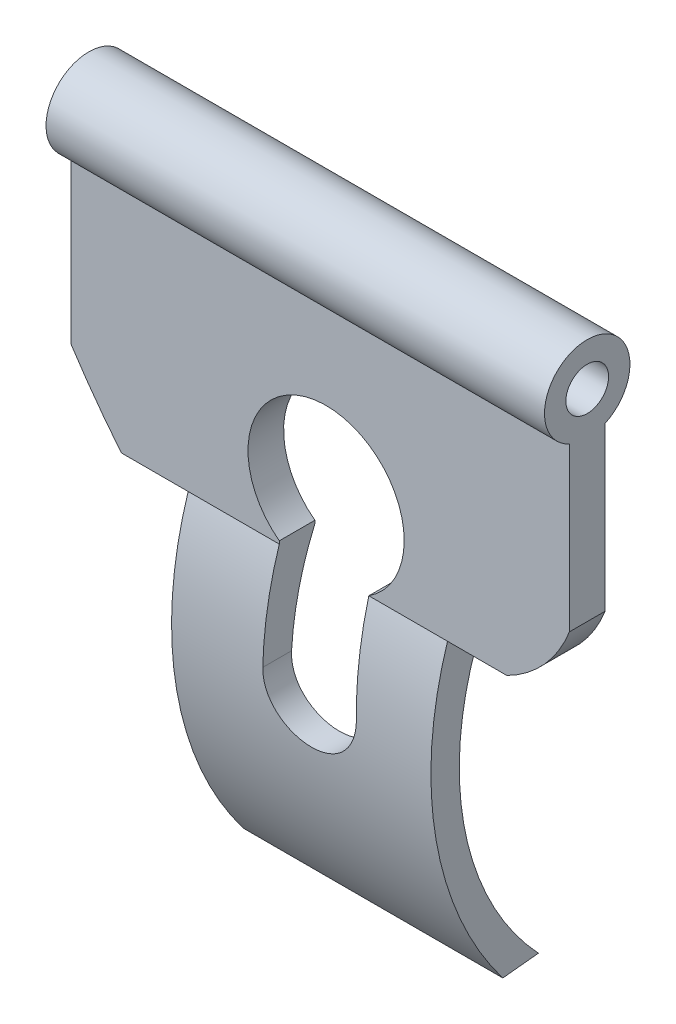
ISO-10303-21;
HEADER;
FILE_DESCRIPTION(('STEP AP214'),'2;1');
FILE_NAME('part.step','',(''),(''),'','','');
FILE_SCHEMA(('AUTOMOTIVE_DESIGN { 1 0 10303 214 1 1 1 1 }'));
ENDSEC;
DATA;
#1=APPLICATION_CONTEXT('core data for automotive mechanical design processes');
#2=APPLICATION_PROTOCOL_DEFINITION('international standard','automotive_design',2000,#1);
#3=PRODUCT_CONTEXT('',#1,'mechanical');
#4=PRODUCT('Part','Part','',(#3));
#5=PRODUCT_RELATED_PRODUCT_CATEGORY('part','',(#4));
#6=PRODUCT_DEFINITION_FORMATION('','',#4);
#7=PRODUCT_DEFINITION_CONTEXT('part definition',#1,'design');
#8=PRODUCT_DEFINITION('design','',#6,#7);
#9=PRODUCT_DEFINITION_SHAPE('','',#8);
#10=(LENGTH_UNIT() NAMED_UNIT(*) SI_UNIT(.MILLI.,.METRE.));
#11=(NAMED_UNIT(*) PLANE_ANGLE_UNIT() SI_UNIT($,.RADIAN.));
#12=(NAMED_UNIT(*) SI_UNIT($,.STERADIAN.) SOLID_ANGLE_UNIT());
#13=UNCERTAINTY_MEASURE_WITH_UNIT(LENGTH_MEASURE(1.E-05),#10,'distance_accuracy_value','');
#14=(GEOMETRIC_REPRESENTATION_CONTEXT(3) GLOBAL_UNCERTAINTY_ASSIGNED_CONTEXT((#13)) GLOBAL_UNIT_ASSIGNED_CONTEXT((#10,
#11,#12)) REPRESENTATION_CONTEXT('',''));
#15=CARTESIAN_POINT('',(0.,0.,0.));
#16=DIRECTION('',(0.,0.,1.));
#17=DIRECTION('',(1.,0.,0.));
#18=AXIS2_PLACEMENT_3D('',#15,#16,#17);
#19=CARTESIAN_POINT('',(6.99999999999999,-52.9712864227578,-44.3974159261056));
#20=DIRECTION('',(1.,0.,0.));
#21=DIRECTION('',(0.,0.,-1.));
#22=AXIS2_PLACEMENT_3D('',#19,#20,#21);
#23=CYLINDRICAL_SURFACE('',#22,49.2291279396497);
#24=CARTESIAN_POINT('',(42.4478068961798,-52.9712864227578,-44.3974159261056));
#25=DIRECTION('',(0.999136886042049,0.0415389329448733,0.));
#26=DIRECTION('',(0.0415389329448733,-0.999136886042049,0.));
#27=AXIS2_PLACEMENT_3D('',#24,#25,#26);
#28=ELLIPSE('',#27,49.2716549928054,49.2291279396497);
#29=CARTESIAN_POINT('',(42.4004064881789,-51.8311633456915,4.81850788994741));
#30=VERTEX_POINT('',#29);
#31=CARTESIAN_POINT('',(41.8253784066492,-38.,2.5));
#32=VERTEX_POINT('',#31);
#33=EDGE_CURVE('E182',#30,#32,#28,.F.);
#34=ORIENTED_EDGE('',*,*,#33,.F.);
#35=CARTESIAN_POINT('',(42.4004064881789,-51.8311633456915,4.81850788994741));
#36=CARTESIAN_POINT('',(42.4004272866516,-52.0148228202435,4.82277278769377));
#37=CARTESIAN_POINT('',(42.3927093008387,-52.1985036306068,4.82598935199668));
#38=CARTESIAN_POINT('',(42.3619341165299,-52.5645884625414,4.83036962650464));
#39=CARTESIAN_POINT('',(42.3388779445284,-52.7469925687296,4.83153347406691));
#40=CARTESIAN_POINT('',(42.2775957275639,-53.1090462090531,4.83185252541183));
#41=CARTESIAN_POINT('',(42.2393850548384,-53.2886983434919,4.8310097603167));
#42=CARTESIAN_POINT('',(42.1480749260284,-53.644156459105,4.82743406908749));
#43=CARTESIAN_POINT('',(42.0949756075018,-53.8199624757978,4.82470116041634));
#44=CARTESIAN_POINT('',(41.9742581345645,-54.1665174469575,4.81750572105998));
#45=CARTESIAN_POINT('',(41.906637220099,-54.3372654330369,4.81304286144073));
#46=CARTESIAN_POINT('',(41.7573422013104,-54.6725294681309,4.80259373184012));
#47=CARTESIAN_POINT('',(41.6756629058677,-54.837043187637,4.79660689873226));
#48=CARTESIAN_POINT('',(41.4988942693706,-55.1585452676515,4.78336094522803));
#49=CARTESIAN_POINT('',(41.4038112649323,-55.3155371374003,4.77610242563115));
#50=CARTESIAN_POINT('',(41.2008420968024,-55.6210450901704,4.76058671666513));
#51=CARTESIAN_POINT('',(41.0929511910275,-55.7695580035581,4.75232915738302));
#52=CARTESIAN_POINT('',(40.8647093433168,-56.0575769758064,4.73508601210607));
#53=CARTESIAN_POINT('',(40.7443116463755,-56.1970458223169,4.72609772372094));
#54=CARTESIAN_POINT('',(40.4922042135143,-56.465423999144,4.70773800860886));
#55=CARTESIAN_POINT('',(40.360490315565,-56.5943294099422,4.69836644158412));
#56=CARTESIAN_POINT('',(40.0867365556308,-56.8406018513904,4.67957143470314));
#57=CARTESIAN_POINT('',(39.9446988003194,-56.9579712246355,4.67014800579052));
#58=CARTESIAN_POINT('',(39.6512082833703,-57.1804235682722,4.65156641941204));
#59=CARTESIAN_POINT('',(39.4997520621253,-57.2855019826076,4.64240836125511));
#60=CARTESIAN_POINT('',(39.1878509828328,-57.4830116330515,4.62463270633958));
#61=CARTESIAN_POINT('',(39.0273699928713,-57.5753860471284,4.61601762558071));
#62=CARTESIAN_POINT('',(38.6990917364206,-57.7463173568394,4.5996604727672));
#63=CARTESIAN_POINT('',(38.5312917779282,-57.8248691139358,4.59191872575443));
#64=CARTESIAN_POINT('',(38.1896957883277,-57.967513154658,4.57757663028869));
#65=CARTESIAN_POINT('',(38.015902492014,-58.0316119351845,4.57097576929753));
#66=CARTESIAN_POINT('',(37.6634195132357,-58.1449479231074,4.55913128898036));
#67=CARTESIAN_POINT('',(37.4847280619881,-58.194179682624,4.55388816728516));
#68=CARTESIAN_POINT('',(37.1244168317102,-58.2772419705253,4.54495441141868));
#69=CARTESIAN_POINT('',(36.9428093788423,-58.3111253962825,4.54125844842583));
#70=CARTESIAN_POINT('',(36.577357970659,-58.3634916039002,4.53551630242693));
#71=CARTESIAN_POINT('',(36.3935139773426,-58.3819741237124,4.53347014749256));
#72=CARTESIAN_POINT('',(36.0249142215589,-58.4033999645648,4.53109618096684));
#73=CARTESIAN_POINT('',(35.8401584720371,-58.4063435055996,4.5307683450482));
#74=CARTESIAN_POINT('',(35.4710601094936,-58.3966700205534,4.53184192656726));
#75=CARTESIAN_POINT('',(35.2867174954444,-58.3840530332211,4.53324333969879));
#76=CARTESIAN_POINT('',(34.9206400396917,-58.3434492359607,4.53771785216521));
#77=CARTESIAN_POINT('',(34.738896974958,-58.3155356332202,4.54078298852421));
#78=CARTESIAN_POINT('',(34.3784227433714,-58.2445940203224,4.54847803563724));
#79=CARTESIAN_POINT('',(34.1996915178474,-58.2015663049481,4.55310791587269));
#80=CARTESIAN_POINT('',(33.8464638134781,-58.1006997626879,4.56378020106195));
#81=CARTESIAN_POINT('',(33.6719681832891,-58.0428579939984,4.56982288655258));
#82=CARTESIAN_POINT('',(33.3285355356356,-57.9128086743332,4.58311758350949));
#83=CARTESIAN_POINT('',(33.1595965372608,-57.8406063089645,4.5903691582937));
#84=CARTESIAN_POINT('',(32.8279446328418,-57.6821255333204,4.60586340056811));
#85=CARTESIAN_POINT('',(32.6652496427565,-57.5958098858852,4.61410867432524));
#86=CARTESIAN_POINT('',(32.3477591459481,-57.4098873761342,4.63129573700929));
#87=CARTESIAN_POINT('',(32.1929607941153,-57.3102853482478,4.64023727210181));
#88=CARTESIAN_POINT('',(31.8922216245507,-57.0984279798047,4.65852198288474));
#89=CARTESIAN_POINT('',(31.7462839968443,-56.9861681232656,4.66786530118074));
#90=CARTESIAN_POINT('',(31.4643920486273,-56.7498511970862,4.6866296035705));
#91=CARTESIAN_POINT('',(31.3284341113722,-56.6257984390994,4.69605055813751));
#92=CARTESIAN_POINT('',(31.0666656532321,-56.3660050605062,4.71470041689289));
#93=CARTESIAN_POINT('',(30.9409154211626,-56.2302035855989,4.72392797053744));
#94=CARTESIAN_POINT('',(30.701338784207,-55.9485123735807,4.7418053591569));
#95=CARTESIAN_POINT('',(30.5875080032234,-55.8026263717834,4.75045540573158));
#96=CARTESIAN_POINT('',(30.3724563320646,-55.501646336587,4.76687030854798));
#97=CARTESIAN_POINT('',(30.2712437324657,-55.3465463470523,4.77463458252535));
#98=CARTESIAN_POINT('',(30.0822783794528,-55.0283789273214,4.78897195642646));
#99=CARTESIAN_POINT('',(29.9945205696038,-54.8653145207552,4.79554550400561));
#100=CARTESIAN_POINT('',(29.8330944341739,-54.5324023606024,4.80723506652109));
#101=CARTESIAN_POINT('',(29.7594192644044,-54.3625579508767,4.81235179007149));
#102=CARTESIAN_POINT('',(29.6266685443386,-54.0172880049236,4.82090102153776));
#103=CARTESIAN_POINT('',(29.5675874145293,-53.8418646306581,4.82433417360352));
#104=CARTESIAN_POINT('',(29.4644758401622,-53.4868264235191,4.82933232381355));
#105=CARTESIAN_POINT('',(29.4204296685412,-53.3072161817153,4.83089927836055));
#106=CARTESIAN_POINT('',(29.3476402120207,-52.9449884342697,4.83203788223034));
#107=CARTESIAN_POINT('',(29.3188895924397,-52.7623724133808,4.83161048886596));
#108=CARTESIAN_POINT('',(29.2836563472731,-52.4546973770444,4.8291583095));
#109=CARTESIAN_POINT('',(29.2729807758379,-52.3300980785225,4.82769402379001));
#110=CARTESIAN_POINT('',(29.2587610500021,-52.0807206316672,4.8238142284511));
#111=CARTESIAN_POINT('',(29.2552048011394,-51.9559431476322,4.8214003403914));
#112=CARTESIAN_POINT('',(29.255207416721,-51.8311633456915,4.8185078899474));
#113=B_SPLINE_CURVE_WITH_KNOTS('',3,(#35,#36,#37,#38,#39,#40,#41,#42,#43,#44,#45,#46,#47,#48,
#49,#50,#51,#52,#53,#54,#55,#56,#57,#58,#59,#60,#61,#62,#63,#64,#65,#66,#67,#68,#69,#70,#71,#72,
#73,#74,#75,#76,#77,#78,#79,#80,#81,#82,#83,#84,#85,#86,#87,#88,#89,#90,#91,#92,#93,#94,#95,#96,
#97,#98,#99,#100,#101,#102,#103,#104,#105,#106,#107,#108,#109,#110,#111,#112),.UNSPECIFIED.,.F.,
.F.,(4,2,2,2,2,2,2,2,2,2,2,2,2,2,2,2,2,2,2,2,2,2,2,2,2,2,2,2,2,2,2,2,2,2,2,2,2,2,4),(0.,
0.550957649228606,1.10187842981338,1.65224179756538,2.2026000806112,2.7530630605223,
3.30372973912141,3.85413695716424,4.4047486010136,4.95749824290263,5.51045206022659,
6.063293357563,6.61633893895976,7.17178286448609,7.72743284066219,8.28283254093139,
8.83843551591308,9.39210878152291,9.94579146775293,10.4994663151433,11.0531397837793,
11.6041863110236,12.1552220913444,12.7063673823802,13.2573140151696,13.8097384706839,
14.3619624645968,14.9143841047404,15.4666045427803,16.0218795128123,16.5769498995431,
17.1323830856685,17.6876070204661,18.2425604254873,18.7973013342543,19.3514601745986,
19.9053530388913,20.2803524190753,20.6547141996082),.UNSPECIFIED.);
#114=CARTESIAN_POINT('',(29.255207416721,-51.8311633456915,4.81850788994741));
#115=VERTEX_POINT('',#114);
#116=EDGE_CURVE('E167',#30,#115,#113,.T.);
#117=ORIENTED_EDGE('',*,*,#116,.T.);
#118=CARTESIAN_POINT('',(29.255207416721,-52.9712864227578,-44.3974159261056));
#119=DIRECTION('',(1.,0.,0.));
#120=DIRECTION('',(0.,0.,-1.));
#121=AXIS2_PLACEMENT_3D('',#118,#119,#120);
#122=CIRCLE('',#121,49.2291279396497);
#123=CARTESIAN_POINT('',(29.255207416721,-38.,2.5));
#124=VERTEX_POINT('',#123);
#125=EDGE_CURVE('E166',#115,#124,#122,.F.);
#126=ORIENTED_EDGE('',*,*,#125,.T.);
#127=DIRECTION('',(-1.,0.,0.));
#128=VECTOR('',#127,1.);
#129=CARTESIAN_POINT('',(70.,-38.,2.5));
#130=LINE('',#129,#128);
#131=CARTESIAN_POINT('',(16.4571242651207,-38.,2.5));
#132=VERTEX_POINT('',#131);
#133=EDGE_CURVE('E170',#124,#132,#130,.T.);
#134=ORIENTED_EDGE('',*,*,#133,.T.);
#135=CARTESIAN_POINT('',(16.4571242651207,-52.9712864227578,-44.3974159261056));
#136=DIRECTION('',(-1.,0.,0.));
#137=DIRECTION('',(0.,0.,1.));
#138=AXIS2_PLACEMENT_3D('',#135,#136,#137);
#139=CIRCLE('',#138,49.2291279396497);
#140=CARTESIAN_POINT('',(16.4571242651207,-82.841381432004,-5.26578598513591));
#141=VERTEX_POINT('',#140);
#142=EDGE_CURVE('E243',#132,#141,#139,.F.);
#143=ORIENTED_EDGE('',*,*,#142,.T.);
#144=DIRECTION('',(1.,0.,0.));
#145=VECTOR('',#144,1.);
#146=CARTESIAN_POINT('',(6.99999999999999,-82.841381432004,-5.26578598513591));
#147=LINE('',#146,#145);
#148=CARTESIAN_POINT('',(52.8806301729192,-82.841381432004,-5.26578598513591));
#149=VERTEX_POINT('',#148);
#150=EDGE_CURVE('E261',#141,#149,#147,.T.);
#151=ORIENTED_EDGE('',*,*,#150,.T.);
#152=CARTESIAN_POINT('',(52.8806301729192,-52.9712864227578,-44.3974159261056));
#153=DIRECTION('',(1.,0.,0.));
#154=DIRECTION('',(0.,0.,-1.));
#155=AXIS2_PLACEMENT_3D('',#152,#153,#154);
#156=CIRCLE('',#155,49.2291279396497);
#157=CARTESIAN_POINT('',(52.8806301729192,-38.,2.49999999999999));
#158=VERTEX_POINT('',#157);
#159=EDGE_CURVE('E256',#149,#158,#156,.F.);
#160=ORIENTED_EDGE('',*,*,#159,.T.);
#161=EDGE_CURVE('E231',#158,#32,#130,.T.);
#162=ORIENTED_EDGE('',*,*,#161,.T.);
#163=EDGE_LOOP('',(#34,#117,#126,#134,#143,#151,#160,#162));
#164=FACE_BOUND('',#163,.T.);
#165=ADVANCED_FACE('F45',(#164),#23,.T.);
#166=CARTESIAN_POINT('',(6.99999999999999,-54.237018869758,-40.2033993287331));
#167=DIRECTION('',(1.,0.,0.));
#168=DIRECTION('',(0.,0.,-1.));
#169=AXIS2_PLACEMENT_3D('',#166,#167,#168);
#170=CYLINDRICAL_SURFACE('',#169,41.0510304708517);
#171=CARTESIAN_POINT('',(42.5004294907178,-54.237018869758,-40.2033993287331));
#172=DIRECTION('',(0.999136886042049,0.0415389329448733,0.));
#173=DIRECTION('',(0.0415389329448733,-0.999136886042049,0.));
#174=AXIS2_PLACEMENT_3D('',#171,#172,#173);
#175=ELLIPSE('',#174,41.0864927962674,41.0510304708517);
#176=CARTESIAN_POINT('',(41.8253784066492,-38.,-2.5));
#177=VERTEX_POINT('',#176);
#178=CARTESIAN_POINT('',(42.4004064881789,-51.8311633456915,0.777071165346227));
#179=VERTEX_POINT('',#178);
#180=EDGE_CURVE('E12',#177,#179,#175,.T.);
#181=ORIENTED_EDGE('',*,*,#180,.F.);
#182=DIRECTION('',(-1.,0.,0.));
#183=VECTOR('',#182,1.);
#184=CARTESIAN_POINT('',(70.,-38.,-2.5));
#185=LINE('',#184,#183);
#186=CARTESIAN_POINT('',(52.8806301729192,-38.,-2.5));
#187=VERTEX_POINT('',#186);
#188=EDGE_CURVE('E314',#187,#177,#185,.T.);
#189=ORIENTED_EDGE('',*,*,#188,.F.);
#190=CARTESIAN_POINT('',(52.8806301729192,-54.237018869758,-40.2033993287331));
#191=DIRECTION('',(1.,0.,0.));
#192=DIRECTION('',(0.,0.,-1.));
#193=AXIS2_PLACEMENT_3D('',#190,#191,#192);
#194=CIRCLE('',#193,41.0510304708517);
#195=CARTESIAN_POINT('',(52.8806301729192,-82.3248527130443,-10.2657859851359));
#196=VERTEX_POINT('',#195);
#197=EDGE_CURVE('E257',#187,#196,#194,.T.);
#198=ORIENTED_EDGE('',*,*,#197,.T.);
#199=DIRECTION('',(1.,0.,0.));
#200=VECTOR('',#199,1.);
#201=CARTESIAN_POINT('',(6.99999999999999,-82.3248527130443,-10.2657859851359));
#202=LINE('',#201,#200);
#203=CARTESIAN_POINT('',(16.4571242651207,-82.3248527130443,-10.2657859851359));
#204=VERTEX_POINT('',#203);
#205=EDGE_CURVE('E265',#204,#196,#202,.T.);
#206=ORIENTED_EDGE('',*,*,#205,.F.);
#207=CARTESIAN_POINT('',(16.4571242651207,-54.237018869758,-40.2033993287331));
#208=DIRECTION('',(-1.,0.,0.));
#209=DIRECTION('',(0.,0.,1.));
#210=AXIS2_PLACEMENT_3D('',#207,#208,#209);
#211=CIRCLE('',#210,41.0510304708517);
#212=CARTESIAN_POINT('',(16.4571242651207,-38.,-2.5));
#213=VERTEX_POINT('',#212);
#214=EDGE_CURVE('E238',#204,#213,#211,.T.);
#215=ORIENTED_EDGE('',*,*,#214,.T.);
#216=CARTESIAN_POINT('',(29.255207416721,-38.,-2.5));
#217=VERTEX_POINT('',#216);
#218=EDGE_CURVE('E311',#217,#213,#185,.T.);
#219=ORIENTED_EDGE('',*,*,#218,.F.);
#220=CARTESIAN_POINT('',(29.255207416721,-54.237018869758,-40.2033993287331));
#221=DIRECTION('',(1.,0.,0.));
#222=DIRECTION('',(0.,0.,-1.));
#223=AXIS2_PLACEMENT_3D('',#220,#221,#222);
#224=CIRCLE('',#223,41.0510304708517);
#225=CARTESIAN_POINT('',(29.255207416721,-51.8311633456915,0.777071165346227));
#226=VERTEX_POINT('',#225);
#227=EDGE_CURVE('E151',#217,#226,#224,.T.);
#228=ORIENTED_EDGE('',*,*,#227,.T.);
#229=CARTESIAN_POINT('',(29.255207416721,-51.8311633456915,0.777071165346227));
#230=CARTESIAN_POINT('',(29.2551862710845,-52.013900503685,0.78781138328913));
#231=CARTESIAN_POINT('',(29.2628275127138,-52.1967096143398,0.797305349333378));
#232=CARTESIAN_POINT('',(29.2933189270613,-52.5611583890662,0.81381167871571));
#233=CARTESIAN_POINT('',(29.3161683031272,-52.7427981138909,0.820824172012072));
#234=CARTESIAN_POINT('',(29.3769285798627,-53.1034267161399,0.832373576017649));
#235=CARTESIAN_POINT('',(29.4148238051525,-53.28241815198,0.836913051578508));
#236=CARTESIAN_POINT('',(29.5054125969348,-53.6366582211059,0.843622917104425));
#237=CARTESIAN_POINT('',(29.5581059482637,-53.8119069087711,0.845793341513061));
#238=CARTESIAN_POINT('',(29.6779396610719,-54.1574584384914,0.847917845102459));
#239=CARTESIAN_POINT('',(29.7450838406128,-54.3277599599303,0.847871337829038));
#240=CARTESIAN_POINT('',(29.8933611044865,-54.6622218276805,0.845769788062237));
#241=CARTESIAN_POINT('',(29.9744993622682,-54.8263798754096,0.84371400144515));
#242=CARTESIAN_POINT('',(30.1501275580187,-55.147253954466,0.83785206132433));
#243=CARTESIAN_POINT('',(30.2446110229159,-55.3039735448552,0.834046754416508));
#244=CARTESIAN_POINT('',(30.4463275536636,-55.6090188799371,0.824981281851952));
#245=CARTESIAN_POINT('',(30.5535653485026,-55.7573414809606,0.819720575604585));
#246=CARTESIAN_POINT('',(30.7803890031573,-56.0449853991545,0.80805215323785));
#247=CARTESIAN_POINT('',(30.9000151196575,-56.1842748165466,0.801640644673474));
#248=CARTESIAN_POINT('',(31.1505215353129,-56.4523902713932,0.788029795262536));
#249=CARTESIAN_POINT('',(31.2814059674549,-56.5812124322238,0.780830164825596));
#250=CARTESIAN_POINT('',(31.553453057285,-56.827423405374,0.766005340486057));
#251=CARTESIAN_POINT('',(31.6946138151236,-56.9448143217266,0.758380225306077));
#252=CARTESIAN_POINT('',(31.9863091073212,-57.1674196595499,0.743057296638023));
#253=CARTESIAN_POINT('',(32.1368470932725,-57.2726295561806,0.7353594572765));
#254=CARTESIAN_POINT('',(32.4472830811458,-57.4707791264487,0.720186094246282));
#255=CARTESIAN_POINT('',(32.6072388571895,-57.5636284526595,0.712712487196203));
#256=CARTESIAN_POINT('',(32.9344863346986,-57.7355630844579,0.698370070397983));
#257=CARTESIAN_POINT('',(33.1017807371311,-57.8146432682162,0.691501486172938));
#258=CARTESIAN_POINT('',(33.4423942049698,-57.9583997671651,0.678670531490853));
#259=CARTESIAN_POINT('',(33.615710561302,-58.0230824647396,0.672707759862171));
#260=CARTESIAN_POINT('',(33.9672751487667,-58.1376424527887,0.66193503747772));
#261=CARTESIAN_POINT('',(34.145525162996,-58.1875143119637,0.657125509753563));
#262=CARTESIAN_POINT('',(34.5053643027338,-58.2719952625799,0.648869509439004));
#263=CARTESIAN_POINT('',(34.6869482088694,-58.306626391512,0.645421069519342));
#264=CARTESIAN_POINT('',(35.0524127875527,-58.3604776304912,0.640020270305216));
#265=CARTESIAN_POINT('',(35.2362935009873,-58.3796974657934,0.638067937682636));
#266=CARTESIAN_POINT('',(35.6050284821548,-58.4025830095945,0.635740122710671));
#267=CARTESIAN_POINT('',(35.7898827400214,-58.4062488754214,0.635364624411638));
#268=CARTESIAN_POINT('',(36.1592393085816,-58.3979997301201,0.636205934242317));
#269=CARTESIAN_POINT('',(36.343741620223,-58.3860847610079,0.637422738078154));
#270=CARTESIAN_POINT('',(36.7102636078965,-58.3468486871214,0.64138965420686));
#271=CARTESIAN_POINT('',(36.8922906271707,-58.3195954488421,0.64413301143375));
#272=CARTESIAN_POINT('',(37.2533895140513,-58.2499318982601,0.651035620126144));
#273=CARTESIAN_POINT('',(37.4324614393567,-58.2075218822654,0.655194843912049));
#274=CARTESIAN_POINT('',(37.7864248537003,-58.1078419353391,0.664758644976362));
#275=CARTESIAN_POINT('',(37.9613154929022,-58.0505690111321,0.670163473085332));
#276=CARTESIAN_POINT('',(38.3055876978027,-57.9216021047379,0.681990937307442));
#277=CARTESIAN_POINT('',(38.4749712309712,-57.8499133400098,0.68841320500543));
#278=CARTESIAN_POINT('',(38.8075294105995,-57.6924135404842,0.702023417913938));
#279=CARTESIAN_POINT('',(38.97068741417,-57.6065675271036,0.709213243625769));
#280=CARTESIAN_POINT('',(39.2891450120115,-57.4215216268564,0.724032215094351));
#281=CARTESIAN_POINT('',(39.4444474485978,-57.3223266181928,0.731661199786547));
#282=CARTESIAN_POINT('',(39.7462296118795,-57.1112155047978,0.747025538856692));
#283=CARTESIAN_POINT('',(39.8927061201492,-56.9992948020074,0.754760930788738));
#284=CARTESIAN_POINT('',(40.1756998498758,-56.7635857505098,0.769976175345955));
#285=CARTESIAN_POINT('',(40.3122207085268,-56.639801774565,0.77745612075947));
#286=CARTESIAN_POINT('',(40.5749846796514,-56.3806218370759,0.791831897448136));
#287=CARTESIAN_POINT('',(40.7011798291845,-56.2451770896073,0.798725008271243));
#288=CARTESIAN_POINT('',(40.941675288446,-55.9641532633959,0.811523342643876));
#289=CARTESIAN_POINT('',(41.0559800066479,-55.8185779742841,0.817428932821558));
#290=CARTESIAN_POINT('',(41.2719962201283,-55.5181829706114,0.827909656277159));
#291=CARTESIAN_POINT('',(41.3736998996042,-55.3633576060434,0.832483966176567));
#292=CARTESIAN_POINT('',(41.5636598666664,-55.0457067379401,0.839972264079861));
#293=CARTESIAN_POINT('',(41.6519212581197,-54.8828843020023,0.842886883404363));
#294=CARTESIAN_POINT('',(41.8141458541011,-54.5508766999773,0.846765919768479));
#295=CARTESIAN_POINT('',(41.8881530735077,-54.3817131122054,0.84773643013108));
#296=CARTESIAN_POINT('',(42.0216514093965,-54.0378261992285,0.847507766434327));
#297=CARTESIAN_POINT('',(42.0811480986328,-53.8631050376386,0.846309426813219));
#298=CARTESIAN_POINT('',(42.1851828875006,-53.5094875947464,0.841564274849871));
#299=CARTESIAN_POINT('',(42.2297357594675,-53.3305956246509,0.838019792098701));
#300=CARTESIAN_POINT('',(42.3036366062835,-52.9698356260756,0.828464936215655));
#301=CARTESIAN_POINT('',(42.3329916827179,-52.7879690286299,0.822455717156139));
#302=CARTESIAN_POINT('',(42.3699134127951,-52.4766731433532,0.810072284142807));
#303=CARTESIAN_POINT('',(42.3813581031596,-52.3476648360665,0.804333180483692));
#304=CARTESIAN_POINT('',(42.3965997019823,-52.0894839051512,0.791623835013054));
#305=CARTESIAN_POINT('',(42.4004099066028,-51.960311959928,0.784655756650464));
#306=CARTESIAN_POINT('',(42.4004064881789,-51.8311633456915,0.777071165346227));
#307=B_SPLINE_CURVE_WITH_KNOTS('',3,(#229,#230,#231,#232,#233,#234,#235,#236,#237,#238,#239,
#240,#241,#242,#243,#244,#245,#246,#247,#248,#249,#250,#251,#252,#253,#254,#255,#256,#257,#258,
#259,#260,#261,#262,#263,#264,#265,#266,#267,#268,#269,#270,#271,#272,#273,#274,#275,#276,#277,
#278,#279,#280,#281,#282,#283,#284,#285,#286,#287,#288,#289,#290,#291,#292,#293,#294,#295,#296,
#297,#298,#299,#300,#301,#302,#303,#304,#305,#306),.UNSPECIFIED.,.F.,.F.,(4,2,2,2,2,2,2,2,2,2,2,
2,2,2,2,2,2,2,2,2,2,2,2,2,2,2,2,2,2,2,2,2,2,2,2,2,2,2,4),(0.,0.548992098899319,1.09795544204003,
1.64634834725046,2.19473327928324,2.74326327867393,3.29199649963299,3.84046446665669,
4.38913642968264,4.93965088569598,5.49036830808905,6.04098417316574,6.5918039217418,
7.14645136521526,7.7013046870533,8.2559115512132,8.81072154547037,9.36472664932581,
9.91874162948923,10.4727510057888,11.0267588881246,11.5783345353855,12.1298994001926,
12.6815754322438,13.2330521569261,13.7859124202628,14.3385711944416,14.8914302941705,
15.4440863899717,15.9991788812913,16.5540648285068,17.1092932392432,17.6643103083577,
18.2175850764174,18.7706470240916,19.323160633827,19.8754158329254,20.2641235305148,
20.6521536672614),.UNSPECIFIED.);
#308=EDGE_CURVE('E49',#226,#179,#307,.T.);
#309=ORIENTED_EDGE('',*,*,#308,.T.);
#310=EDGE_LOOP('',(#181,#189,#198,#206,#215,#219,#228,#309));
#311=FACE_BOUND('',#310,.T.);
#312=ADVANCED_FACE('F207',(#311),#170,.F.);
#313=CARTESIAN_POINT('',(6.99999999999999,-82.841381432004,-5.26578598513591));
#314=DIRECTION('',(0.,-0.994706295284288,-0.102758873688879));
#315=DIRECTION('',(0.,0.102758873688879,-0.994706295284288));
#316=AXIS2_PLACEMENT_3D('',#313,#314,#315);
#317=PLANE('',#316);
#318=ORIENTED_EDGE('',*,*,#150,.F.);
#319=DIRECTION('',(0.,0.102758873688879,-0.994706295284288));
#320=VECTOR('',#319,1.);
#321=CARTESIAN_POINT('',(16.4571242651207,-82.841381432004,-5.26578598513591));
#322=LINE('',#321,#320);
#323=EDGE_CURVE('E321',#141,#204,#322,.T.);
#324=ORIENTED_EDGE('',*,*,#323,.T.);
#325=ORIENTED_EDGE('',*,*,#205,.T.);
#326=DIRECTION('',(0.,-0.102758873688879,0.994706295284288));
#327=VECTOR('',#326,1.);
#328=CARTESIAN_POINT('',(52.8806301729192,-82.841381432004,-5.26578598513591));
#329=LINE('',#328,#327);
#330=EDGE_CURVE('E322',#196,#149,#329,.T.);
#331=ORIENTED_EDGE('',*,*,#330,.T.);
#332=EDGE_LOOP('',(#318,#324,#325,#331));
#333=FACE_BOUND('',#332,.T.);
#334=ADVANCED_FACE('F208',(#333),#317,.T.);
#335=CARTESIAN_POINT('',(70.,0.,0.));
#336=DIRECTION('',(1.,0.,0.));
#337=DIRECTION('',(0.,0.,-1.));
#338=AXIS2_PLACEMENT_3D('',#335,#336,#337);
#339=PLANE('',#338);
#340=DIRECTION('',(0.,0.,-1.));
#341=VECTOR('',#340,1.);
#342=CARTESIAN_POINT('',(70.,-28.2978126777009,67.5));
#343=LINE('',#342,#341);
#344=CARTESIAN_POINT('',(70.,-28.2978126777009,2.5));
#345=VERTEX_POINT('',#344);
#346=CARTESIAN_POINT('',(70.,-28.2978126777009,-2.5));
#347=VERTEX_POINT('',#346);
#348=EDGE_CURVE('E270',#345,#347,#343,.T.);
#349=ORIENTED_EDGE('',*,*,#348,.T.);
#350=DIRECTION('',(0.,1.,0.));
#351=VECTOR('',#350,1.);
#352=CARTESIAN_POINT('',(70.,-5.45435605731786,-2.5));
#353=LINE('',#352,#351);
#354=CARTESIAN_POINT('',(70.,-5.45435605731786,-2.5));
#355=VERTEX_POINT('',#354);
#356=EDGE_CURVE('E297',#347,#355,#353,.T.);
#357=ORIENTED_EDGE('',*,*,#356,.T.);
#358=CARTESIAN_POINT('',(70.,0.,0.));
#359=DIRECTION('',(1.,0.,0.));
#360=DIRECTION('',(0.,0.,-1.));
#361=AXIS2_PLACEMENT_3D('',#358,#359,#360);
#362=CIRCLE('',#361,6.);
#363=CARTESIAN_POINT('',(70.,-5.45435605731786,2.5));
#364=VERTEX_POINT('',#363);
#365=EDGE_CURVE('E291',#355,#364,#362,.T.);
#366=ORIENTED_EDGE('',*,*,#365,.T.);
#367=DIRECTION('',(0.,-1.,0.));
#368=VECTOR('',#367,1.);
#369=CARTESIAN_POINT('',(70.,-5.45435605731786,2.5));
#370=LINE('',#369,#368);
#371=EDGE_CURVE('E298',#364,#345,#370,.T.);
#372=ORIENTED_EDGE('',*,*,#371,.T.);
#373=EDGE_LOOP('',(#349,#357,#366,#372));
#374=FACE_BOUND('',#373,.T.);
#375=CARTESIAN_POINT('',(70.,0.,0.));
#376=DIRECTION('',(1.,0.,0.));
#377=DIRECTION('',(0.,0.,-1.));
#378=AXIS2_PLACEMENT_3D('',#375,#376,#377);
#379=CIRCLE('',#378,3.);
#380=CARTESIAN_POINT('',(70.,0.,-3.));
#381=VERTEX_POINT('',#380);
#382=EDGE_CURVE('E286',#381,#381,#379,.T.);
#383=ORIENTED_EDGE('',*,*,#382,.F.);
#384=EDGE_LOOP('',(#383));
#385=FACE_BOUND('',#384,.T.);
#386=ADVANCED_FACE('F213',(#374,#385),#339,.T.);
#387=CARTESIAN_POINT('',(0.,0.,0.));
#388=DIRECTION('',(1.,0.,0.));
#389=DIRECTION('',(0.,0.,-1.));
#390=AXIS2_PLACEMENT_3D('',#387,#388,#389);
#391=PLANE('',#390);
#392=DIRECTION('',(0.,1.,0.));
#393=VECTOR('',#392,1.);
#394=CARTESIAN_POINT('',(0.,-5.45435605731786,-2.5));
#395=LINE('',#394,#393);
#396=CARTESIAN_POINT('',(0.,-28.2978126777009,-2.5));
#397=VERTEX_POINT('',#396);
#398=CARTESIAN_POINT('',(0.,-5.45435605731786,-2.5));
#399=VERTEX_POINT('',#398);
#400=EDGE_CURVE('E300',#397,#399,#395,.T.);
#401=ORIENTED_EDGE('',*,*,#400,.F.);
#402=DIRECTION('',(0.,0.,-1.));
#403=VECTOR('',#402,1.);
#404=CARTESIAN_POINT('',(0.,-28.2978126777009,67.5));
#405=LINE('',#404,#403);
#406=CARTESIAN_POINT('',(0.,-28.2978126777009,2.5));
#407=VERTEX_POINT('',#406);
#408=EDGE_CURVE('E268',#407,#397,#405,.T.);
#409=ORIENTED_EDGE('',*,*,#408,.F.);
#410=DIRECTION('',(0.,-1.,0.));
#411=VECTOR('',#410,1.);
#412=CARTESIAN_POINT('',(0.,-5.45435605731786,2.5));
#413=LINE('',#412,#411);
#414=CARTESIAN_POINT('',(0.,-5.45435605731786,2.5));
#415=VERTEX_POINT('',#414);
#416=EDGE_CURVE('E304',#415,#407,#413,.T.);
#417=ORIENTED_EDGE('',*,*,#416,.F.);
#418=CARTESIAN_POINT('',(0.,0.,0.));
#419=DIRECTION('',(1.,0.,0.));
#420=DIRECTION('',(0.,0.,-1.));
#421=AXIS2_PLACEMENT_3D('',#418,#419,#420);
#422=CIRCLE('',#421,6.);
#423=EDGE_CURVE('E287',#399,#415,#422,.T.);
#424=ORIENTED_EDGE('',*,*,#423,.F.);
#425=EDGE_LOOP('',(#401,#409,#417,#424));
#426=FACE_BOUND('',#425,.T.);
#427=CARTESIAN_POINT('',(0.,0.,0.));
#428=DIRECTION('',(1.,0.,0.));
#429=DIRECTION('',(0.,0.,-1.));
#430=AXIS2_PLACEMENT_3D('',#427,#428,#429);
#431=CIRCLE('',#430,3.);
#432=CARTESIAN_POINT('',(0.,0.,-3.));
#433=VERTEX_POINT('',#432);
#434=EDGE_CURVE('E289',#433,#433,#431,.T.);
#435=ORIENTED_EDGE('',*,*,#434,.T.);
#436=EDGE_LOOP('',(#435));
#437=FACE_BOUND('',#436,.T.);
#438=ADVANCED_FACE('F221',(#426,#437),#391,.F.);
#439=CARTESIAN_POINT('',(70.,0.,0.));
#440=DIRECTION('',(-1.,0.,0.));
#441=DIRECTION('',(0.,0.,1.));
#442=AXIS2_PLACEMENT_3D('',#439,#440,#441);
#443=CYLINDRICAL_SURFACE('',#442,6.);
#444=ORIENTED_EDGE('',*,*,#423,.T.);
#445=DIRECTION('',(-1.,0.,0.));
#446=VECTOR('',#445,1.);
#447=CARTESIAN_POINT('',(70.,-5.45435605731786,2.5));
#448=LINE('',#447,#446);
#449=EDGE_CURVE('E319',#364,#415,#448,.T.);
#450=ORIENTED_EDGE('',*,*,#449,.F.);
#451=ORIENTED_EDGE('',*,*,#365,.F.);
#452=DIRECTION('',(-1.,0.,0.));
#453=VECTOR('',#452,1.);
#454=CARTESIAN_POINT('',(70.,-5.45435605731786,-2.5));
#455=LINE('',#454,#453);
#456=EDGE_CURVE('E305',#355,#399,#455,.T.);
#457=ORIENTED_EDGE('',*,*,#456,.T.);
#458=EDGE_LOOP('',(#444,#450,#451,#457));
#459=FACE_BOUND('',#458,.T.);
#460=ADVANCED_FACE('F42',(#459),#443,.T.);
#461=CARTESIAN_POINT('',(70.,-5.45435605731786,2.5));
#462=DIRECTION('',(0.,0.,-1.));
#463=DIRECTION('',(0.,1.,0.));
#464=AXIS2_PLACEMENT_3D('',#461,#462,#463);
#465=PLANE('',#464);
#466=DIRECTION('',(0.,-1.,0.));
#467=VECTOR('',#466,1.);
#468=CARTESIAN_POINT('',(29.255207416721,-5.45435605731786,2.5));
#469=LINE('',#468,#467);
#470=CARTESIAN_POINT('',(29.255207416721,-37.5975682128737,2.5));
#471=VERTEX_POINT('',#470);
#472=EDGE_CURVE('E156',#471,#124,#469,.T.);
#473=ORIENTED_EDGE('',*,*,#472,.F.);
#474=CARTESIAN_POINT('',(35.8278069524499,-28.8181300675824,2.5));
#475=DIRECTION('',(0.,0.,-1.));
#476=DIRECTION('',(0.,1.,0.));
#477=AXIS2_PLACEMENT_3D('',#474,#475,#476);
#478=CIRCLE('',#477,10.9671144246817);
#479=EDGE_CURVE('E143',#32,#471,#478,.F.);
#480=ORIENTED_EDGE('',*,*,#479,.F.);
#481=ORIENTED_EDGE('',*,*,#161,.F.);
#482=CARTESIAN_POINT('',(61.2084532475594,-38.,2.49999999999999));
#483=VERTEX_POINT('',#482);
#484=EDGE_CURVE('E317',#483,#158,#130,.T.);
#485=ORIENTED_EDGE('',*,*,#484,.F.);
#486=CARTESIAN_POINT('',(53.0131562371972,-21.7396250819844,2.5));
#487=DIRECTION('',(0.,0.,-1.));
#488=DIRECTION('',(0.,1.,0.));
#489=AXIS2_PLACEMENT_3D('',#486,#487,#488);
#490=CIRCLE('',#489,18.20886283002);
#491=EDGE_CURVE('E282',#483,#345,#490,.F.);
#492=ORIENTED_EDGE('',*,*,#491,.T.);
#493=ORIENTED_EDGE('',*,*,#371,.F.);
#494=ORIENTED_EDGE('',*,*,#449,.T.);
#495=ORIENTED_EDGE('',*,*,#416,.T.);
#496=CARTESIAN_POINT('',(93.2418704895458,32.2909532219158,2.5));
#497=DIRECTION('',(0.,0.,-1.));
#498=DIRECTION('',(0.,1.,0.));
#499=AXIS2_PLACEMENT_3D('',#496,#497,#498);
#500=CIRCLE('',#499,111.198223752126);
#501=CARTESIAN_POINT('',(7.07791711702326,-38.,2.5));
#502=VERTEX_POINT('',#501);
#503=EDGE_CURVE('E271',#407,#502,#500,.F.);
#504=ORIENTED_EDGE('',*,*,#503,.T.);
#505=DIRECTION('',(1.,0.,0.));
#506=VECTOR('',#505,1.);
#507=CARTESIAN_POINT('',(70.,-38.,2.5));
#508=LINE('',#507,#506);
#509=EDGE_CURVE('E251',#502,#132,#508,.T.);
#510=ORIENTED_EDGE('',*,*,#509,.T.);
#511=ORIENTED_EDGE('',*,*,#133,.F.);
#512=EDGE_LOOP('',(#473,#480,#481,#485,#492,#493,#494,#495,#504,#510,#511));
#513=FACE_BOUND('',#512,.T.);
#514=ADVANCED_FACE('F164',(#513),#465,.F.);
#515=CARTESIAN_POINT('',(70.,-5.45435605731786,-2.5));
#516=DIRECTION('',(0.,0.,1.));
#517=DIRECTION('',(0.,-1.,0.));
#518=AXIS2_PLACEMENT_3D('',#515,#516,#517);
#519=PLANE('',#518);
#520=DIRECTION('',(0.,1.,0.));
#521=VECTOR('',#520,1.);
#522=CARTESIAN_POINT('',(29.255207416721,-5.45435605731786,-2.5));
#523=LINE('',#522,#521);
#524=CARTESIAN_POINT('',(29.255207416721,-37.5975682128737,-2.5));
#525=VERTEX_POINT('',#524);
#526=EDGE_CURVE('E157',#217,#525,#523,.T.);
#527=ORIENTED_EDGE('',*,*,#526,.F.);
#528=ORIENTED_EDGE('',*,*,#218,.T.);
#529=DIRECTION('',(1.,0.,0.));
#530=VECTOR('',#529,1.);
#531=CARTESIAN_POINT('',(6.99999999999999,-38.,-2.5));
#532=LINE('',#531,#530);
#533=CARTESIAN_POINT('',(7.07791711702327,-38.,-2.5));
#534=VERTEX_POINT('',#533);
#535=EDGE_CURVE('E252',#534,#213,#532,.T.);
#536=ORIENTED_EDGE('',*,*,#535,.F.);
#537=CARTESIAN_POINT('',(93.2418704895458,32.2909532219158,-2.49999999999999));
#538=DIRECTION('',(0.,0.,1.));
#539=DIRECTION('',(0.,1.,0.));
#540=AXIS2_PLACEMENT_3D('',#537,#538,#539);
#541=CIRCLE('',#540,111.198223752126);
#542=EDGE_CURVE('E263',#397,#534,#541,.T.);
#543=ORIENTED_EDGE('',*,*,#542,.F.);
#544=ORIENTED_EDGE('',*,*,#400,.T.);
#545=ORIENTED_EDGE('',*,*,#456,.F.);
#546=ORIENTED_EDGE('',*,*,#356,.F.);
#547=CARTESIAN_POINT('',(53.0131562371972,-21.7396250819844,-2.5));
#548=DIRECTION('',(0.,0.,1.));
#549=DIRECTION('',(0.,1.,0.));
#550=AXIS2_PLACEMENT_3D('',#547,#548,#549);
#551=CIRCLE('',#550,18.20886283002);
#552=CARTESIAN_POINT('',(61.2084532475594,-38.,-2.5));
#553=VERTEX_POINT('',#552);
#554=EDGE_CURVE('E269',#553,#347,#551,.T.);
#555=ORIENTED_EDGE('',*,*,#554,.F.);
#556=EDGE_CURVE('E315',#553,#187,#185,.T.);
#557=ORIENTED_EDGE('',*,*,#556,.T.);
#558=ORIENTED_EDGE('',*,*,#188,.T.);
#559=CARTESIAN_POINT('',(35.8278069524499,-28.8181300675824,-2.5));
#560=DIRECTION('',(0.,0.,1.));
#561=DIRECTION('',(0.,-1.,0.));
#562=AXIS2_PLACEMENT_3D('',#559,#560,#561);
#563=CIRCLE('',#562,10.9671144246817);
#564=EDGE_CURVE('E326',#525,#177,#563,.F.);
#565=ORIENTED_EDGE('',*,*,#564,.F.);
#566=EDGE_LOOP('',(#527,#528,#536,#543,#544,#545,#546,#555,#557,#558,#565));
#567=FACE_BOUND('',#566,.T.);
#568=ADVANCED_FACE('F335',(#567),#519,.F.);
#569=CARTESIAN_POINT('',(70.,0.,0.));
#570=DIRECTION('',(-1.,0.,0.));
#571=DIRECTION('',(0.,0.,1.));
#572=AXIS2_PLACEMENT_3D('',#569,#570,#571);
#573=CYLINDRICAL_SURFACE('',#572,3.);
#574=ORIENTED_EDGE('',*,*,#382,.T.);
#575=EDGE_LOOP('',(#574));
#576=FACE_BOUND('',#575,.T.);
#577=ORIENTED_EDGE('',*,*,#434,.F.);
#578=EDGE_LOOP('',(#577));
#579=FACE_BOUND('',#578,.T.);
#580=ADVANCED_FACE('F385',(#576,#579),#573,.F.);
#581=CARTESIAN_POINT('',(93.2418704895458,32.2909532219158,67.5));
#582=DIRECTION('',(0.,0.,-1.));
#583=DIRECTION('',(0.,1.,0.));
#584=AXIS2_PLACEMENT_3D('',#581,#582,#583);
#585=CYLINDRICAL_SURFACE('',#584,111.198223752126);
#586=ORIENTED_EDGE('',*,*,#408,.T.);
#587=ORIENTED_EDGE('',*,*,#542,.T.);
#588=DIRECTION('',(0.,0.,-1.));
#589=VECTOR('',#588,1.);
#590=CARTESIAN_POINT('',(7.07791711702327,-38.,67.5));
#591=LINE('',#590,#589);
#592=EDGE_CURVE('E279',#502,#534,#591,.T.);
#593=ORIENTED_EDGE('',*,*,#592,.F.);
#594=ORIENTED_EDGE('',*,*,#503,.F.);
#595=EDGE_LOOP('',(#586,#587,#593,#594));
#596=FACE_BOUND('',#595,.T.);
#597=ADVANCED_FACE('F345',(#596),#585,.T.);
#598=CARTESIAN_POINT('',(53.0131562371972,-21.7396250819844,67.5));
#599=DIRECTION('',(0.,0.,-1.));
#600=DIRECTION('',(0.,1.,0.));
#601=AXIS2_PLACEMENT_3D('',#598,#599,#600);
#602=CYLINDRICAL_SURFACE('',#601,18.20886283002);
#603=DIRECTION('',(0.,0.,-1.));
#604=VECTOR('',#603,1.);
#605=CARTESIAN_POINT('',(61.2084532475594,-38.,67.5));
#606=LINE('',#605,#604);
#607=EDGE_CURVE('E267',#483,#553,#606,.T.);
#608=ORIENTED_EDGE('',*,*,#607,.T.);
#609=ORIENTED_EDGE('',*,*,#554,.T.);
#610=ORIENTED_EDGE('',*,*,#348,.F.);
#611=ORIENTED_EDGE('',*,*,#491,.F.);
#612=EDGE_LOOP('',(#608,#609,#610,#611));
#613=FACE_BOUND('',#612,.T.);
#614=ADVANCED_FACE('F352',(#613),#602,.T.);
#615=CARTESIAN_POINT('',(0.,-38.,63.));
#616=DIRECTION('',(0.,1.,0.));
#617=DIRECTION('',(0.,0.,1.));
#618=AXIS2_PLACEMENT_3D('',#615,#616,#617);
#619=PLANE('',#618);
#620=ORIENTED_EDGE('',*,*,#484,.T.);
#621=DIRECTION('',(0.,0.,-1.));
#622=VECTOR('',#621,1.);
#623=CARTESIAN_POINT('',(52.8806301729192,-38.,63.));
#624=LINE('',#623,#622);
#625=EDGE_CURVE('E247',#158,#187,#624,.T.);
#626=ORIENTED_EDGE('',*,*,#625,.T.);
#627=ORIENTED_EDGE('',*,*,#556,.F.);
#628=ORIENTED_EDGE('',*,*,#607,.F.);
#629=EDGE_LOOP('',(#620,#626,#627,#628));
#630=FACE_BOUND('',#629,.T.);
#631=ADVANCED_FACE('F215',(#630),#619,.F.);
#632=CARTESIAN_POINT('',(52.8806301729192,0.,63.));
#633=DIRECTION('',(1.,0.,0.));
#634=DIRECTION('',(0.,0.,-1.));
#635=AXIS2_PLACEMENT_3D('',#632,#633,#634);
#636=PLANE('',#635);
#637=ORIENTED_EDGE('',*,*,#330,.F.);
#638=ORIENTED_EDGE('',*,*,#197,.F.);
#639=ORIENTED_EDGE('',*,*,#625,.F.);
#640=ORIENTED_EDGE('',*,*,#159,.F.);
#641=EDGE_LOOP('',(#637,#638,#639,#640));
#642=FACE_BOUND('',#641,.T.);
#643=ADVANCED_FACE('F361',(#642),#636,.T.);
#644=CARTESIAN_POINT('',(0.,-38.,63.));
#645=DIRECTION('',(0.,1.,0.));
#646=DIRECTION('',(0.,0.,1.));
#647=AXIS2_PLACEMENT_3D('',#644,#645,#646);
#648=PLANE('',#647);
#649=DIRECTION('',(0.,0.,-1.));
#650=VECTOR('',#649,1.);
#651=CARTESIAN_POINT('',(16.4571242651207,-38.,63.));
#652=LINE('',#651,#650);
#653=EDGE_CURVE('E236',#132,#213,#652,.T.);
#654=ORIENTED_EDGE('',*,*,#653,.F.);
#655=ORIENTED_EDGE('',*,*,#509,.F.);
#656=ORIENTED_EDGE('',*,*,#592,.T.);
#657=ORIENTED_EDGE('',*,*,#535,.T.);
#658=EDGE_LOOP('',(#654,#655,#656,#657));
#659=FACE_BOUND('',#658,.T.);
#660=ADVANCED_FACE('F339',(#659),#648,.F.);
#661=CARTESIAN_POINT('',(16.4571242651207,-38.,63.));
#662=DIRECTION('',(-1.,0.,0.));
#663=DIRECTION('',(0.,0.,1.));
#664=AXIS2_PLACEMENT_3D('',#661,#662,#663);
#665=PLANE('',#664);
#666=ORIENTED_EDGE('',*,*,#653,.T.);
#667=ORIENTED_EDGE('',*,*,#214,.F.);
#668=ORIENTED_EDGE('',*,*,#323,.F.);
#669=ORIENTED_EDGE('',*,*,#142,.F.);
#670=EDGE_LOOP('',(#666,#667,#668,#669));
#671=FACE_BOUND('',#670,.T.);
#672=ADVANCED_FACE('F368',(#671),#665,.T.);
#673=CARTESIAN_POINT('',(35.8278069524499,-28.8181300675824,-65.5));
#674=DIRECTION('',(0.,0.,1.));
#675=DIRECTION('',(0.,-1.,0.));
#676=AXIS2_PLACEMENT_3D('',#673,#674,#675);
#677=CYLINDRICAL_SURFACE('',#676,10.9671144246817);
#678=ORIENTED_EDGE('',*,*,#479,.T.);
#679=DIRECTION('',(0.,0.,1.));
#680=VECTOR('',#679,1.);
#681=CARTESIAN_POINT('',(29.255207416721,-37.5975682128737,-65.5));
#682=LINE('',#681,#680);
#683=EDGE_CURVE('E65',#525,#471,#682,.T.);
#684=ORIENTED_EDGE('',*,*,#683,.F.);
#685=ORIENTED_EDGE('',*,*,#564,.T.);
#686=DIRECTION('',(0.,0.,1.));
#687=VECTOR('',#686,1.);
#688=CARTESIAN_POINT('',(41.8253784066492,-38.,-65.5));
#689=LINE('',#688,#687);
#690=EDGE_CURVE('E60',#177,#32,#689,.T.);
#691=ORIENTED_EDGE('',*,*,#690,.T.);
#692=EDGE_LOOP('',(#678,#684,#685,#691));
#693=FACE_BOUND('',#692,.T.);
#694=ADVANCED_FACE('F147',(#693),#677,.F.);
#695=CARTESIAN_POINT('',(40.1760923850651,1.67031367862044,-65.5));
#696=DIRECTION('',(0.999136886042049,0.0415389329448733,0.));
#697=DIRECTION('',(-0.0415389329448733,0.999136886042049,0.));
#698=AXIS2_PLACEMENT_3D('',#695,#696,#697);
#699=PLANE('',#698);
#700=ORIENTED_EDGE('',*,*,#33,.T.);
#701=ORIENTED_EDGE('',*,*,#690,.F.);
#702=ORIENTED_EDGE('',*,*,#180,.T.);
#703=DIRECTION('',(0.,0.,1.));
#704=VECTOR('',#703,1.);
#705=CARTESIAN_POINT('',(42.4004064881789,-51.8311633456915,-65.5));
#706=LINE('',#705,#704);
#707=EDGE_CURVE('E155',#179,#30,#706,.T.);
#708=ORIENTED_EDGE('',*,*,#707,.T.);
#709=EDGE_LOOP('',(#700,#701,#702,#708));
#710=FACE_BOUND('',#709,.T.);
#711=ADVANCED_FACE('F194',(#710),#699,.F.);
#712=CARTESIAN_POINT('',(35.8278069524499,-51.8311633456915,-65.5));
#713=DIRECTION('',(0.,0.,1.));
#714=DIRECTION('',(0.,-1.,0.));
#715=AXIS2_PLACEMENT_3D('',#712,#713,#714);
#716=CYLINDRICAL_SURFACE('',#715,6.57259953572896);
#717=ORIENTED_EDGE('',*,*,#707,.F.);
#718=ORIENTED_EDGE('',*,*,#308,.F.);
#719=DIRECTION('',(0.,0.,1.));
#720=VECTOR('',#719,1.);
#721=CARTESIAN_POINT('',(29.255207416721,-51.8311633456915,-65.5));
#722=LINE('',#721,#720);
#723=EDGE_CURVE('E162',#226,#115,#722,.T.);
#724=ORIENTED_EDGE('',*,*,#723,.T.);
#725=ORIENTED_EDGE('',*,*,#116,.F.);
#726=EDGE_LOOP('',(#717,#718,#724,#725));
#727=FACE_BOUND('',#726,.T.);
#728=ADVANCED_FACE('F189',(#727),#716,.F.);
#729=CARTESIAN_POINT('',(29.255207416721,0.,-65.5));
#730=DIRECTION('',(1.,0.,0.));
#731=DIRECTION('',(0.,0.,-1.));
#732=AXIS2_PLACEMENT_3D('',#729,#730,#731);
#733=PLANE('',#732);
#734=ORIENTED_EDGE('',*,*,#723,.F.);
#735=ORIENTED_EDGE('',*,*,#227,.F.);
#736=ORIENTED_EDGE('',*,*,#526,.T.);
#737=ORIENTED_EDGE('',*,*,#683,.T.);
#738=ORIENTED_EDGE('',*,*,#472,.T.);
#739=ORIENTED_EDGE('',*,*,#125,.F.);
#740=EDGE_LOOP('',(#734,#735,#736,#737,#738,#739));
#741=FACE_BOUND('',#740,.T.);
#742=ADVANCED_FACE('F159',(#741),#733,.T.);
#743=CLOSED_SHELL('',(#165,#312,#334,#386,#438,#460,#514,#568,#580,#597,#614,#631,#643,#660,
#672,#694,#711,#728,#742));
#744=MANIFOLD_SOLID_BREP('B2',#743);
#745=ADVANCED_BREP_SHAPE_REPRESENTATION('',(#18,#744),#14);
#746=SHAPE_DEFINITION_REPRESENTATION(#9,#745);
ENDSEC;
END-ISO-10303-21;
